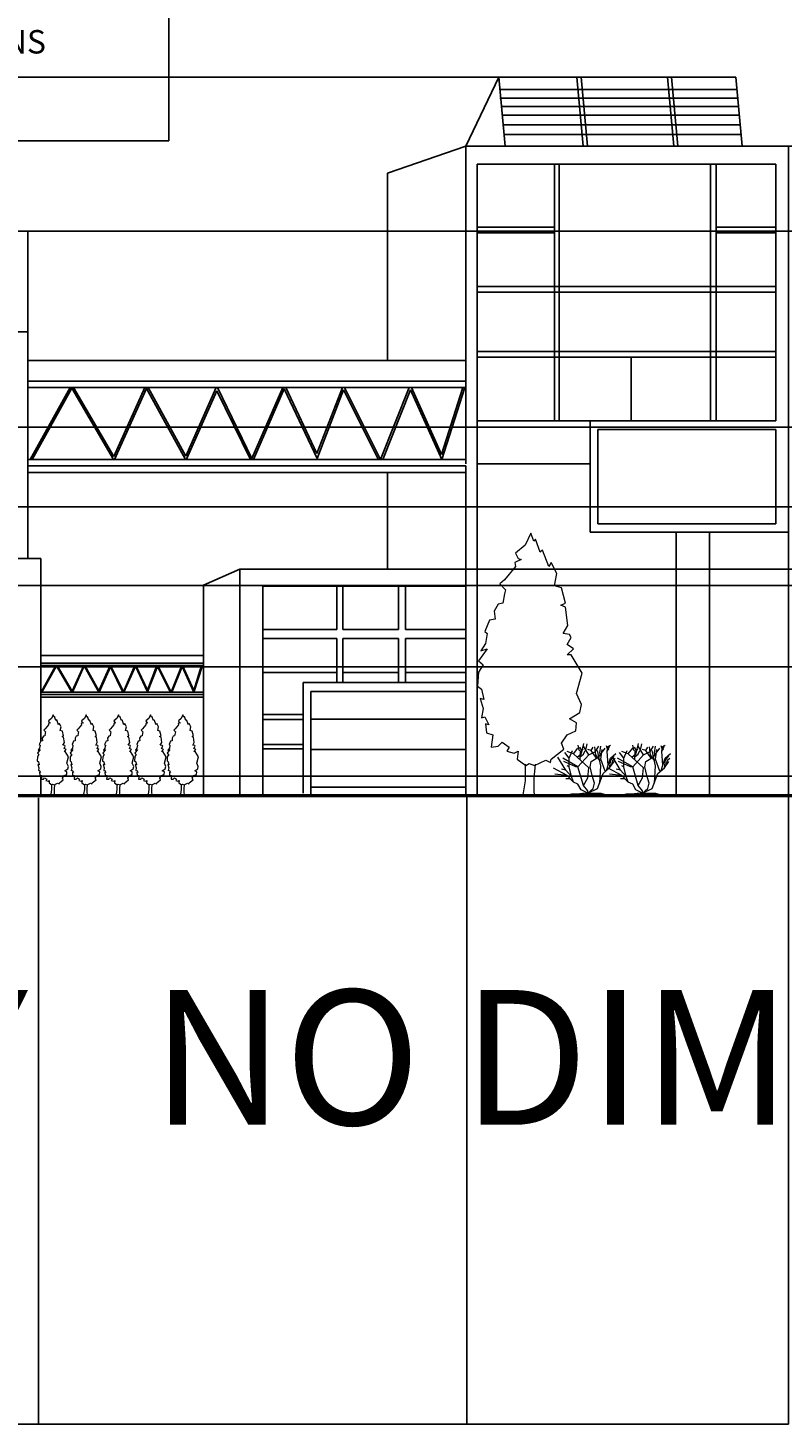
# Model space of a CAD drawing. Units: inches. Extents: x -32109 to 33221, y -19197 to 7608.
# Tile 17 of 25: x 2967 to 6939, y -5430 to 1922. Entities that reach past the tile are written whole.
import ezdxf

# ---------------------------------------------------------------- set-up
doc = ezdxf.new("R2010")
doc.units = ezdxf.units.IN
doc.header["$MEASUREMENT"] = 0
for name, color, linetype, lineweight in [('A-ANNO-DIMS', 2, 'Continuous', 18), ('A-ANNO-TEXT', 7, 'Continuous', 25), ('A-ELEV', 7, 'Continuous', 25), ('L-PLNT', 3, 'Continuous', 13)]:
    doc.layers.add(name, color=color, linetype=linetype, lineweight=lineweight)
doc.styles.get("Standard").update_dxf_attribs({"font": 'arial.ttf'})
doc.dimstyles.get("Standard").update_dxf_attribs({"dimtxt": 0.18, "dimasz": 0.18, "dimexe": 0.18, "dimexo": 0.0625, "dimgap": 0.09, "dimtad": 0, "dimtih": 1, "dimtoh": 1, "dimdec": 4, "dimzin": 0, "dimdsep": 46, "dimtxsty": 'Standard', "dimcen": 0.09, "dimadec": 0, "dimazin": 0, "dimtfac": 1, "dimtdec": 4, "dimtofl": 0, "dimtmove": 0, "dimatfit": 3, "dimfxl": 1, "dimtolj": 1, "dimtzin": 0, "dimarcsym": 0})

# ---------------------------------------------------------------- blocks, each defined once
blk = doc.blocks.new('*U2')
blk.add_lwpolyline([(-2.75400000000036, 191.699), (-6.7800000000002, 182.8509999999996), (-13.68200000000024, 176.9529999999995), (-11.95600000000013, 173.2659999999996), (-9.655999999999949, 172.529), (-14.25700000000006, 170.317), (-13.68200000000024, 167.3679999999999), (-21.73300000000017, 157.7829999999999), (-25.1840000000002, 154.8340000000003), (-21.15800000000036, 150.4099999999998), (-21.73300000000017, 147.4609999999998), (-22.88400000000001, 140.8249999999998), (-26.33400000000029, 140.087), (-29.21000000000004, 134.9259999999995), (-28.63499999999977, 129.0279999999998), (-32.66100000000006, 128.2909999999997), (-36.11099999999988, 120.1799999999998), (-34.38599999999997, 118.7059999999997), (-35.53600000000006, 111.3329999999996), (-38.98700000000008, 106.1709999999998), (-34.38599999999997, 107.6459999999997), (-40.71199999999999, 98.79799999999977), (-37.26099999999997, 95.8489999999997), (-40.71199999999999, 90.68799999999965), (-41.28700000000026, 80.36599999999999), (-38.41200000000026, 78.154), (-36.68600000000015, 70.78099999999995), (-39.5619999999999, 71.51799999999957), (-37.26099999999997, 64.14499999999998), (-38.41200000000026, 57.50899999999956), (-36.11099999999988, 58.24699999999984), (-33.23599999999988, 52.3479999999995), (-35.53600000000006, 53.08599999999978), (-34.96100000000024, 46.44999999999981), (-30.36000000000013, 44.9749999999999), (-31.50999999999977, 36.1279999999997), (-26.33400000000029, 36.86499999999978), (-23.45900000000029, 39.81399999999985), (-18.28300000000036, 36.1279999999997), (-20.00800000000027, 33.17799999999988), (-14.83199999999988, 31.70399999999972), (-11.95600000000013, 33.17799999999988), (-12.53099999999995, 27.27999999999975), (-6.204999999999927, 22.85599999999977), (-3.9050000000002, 24.33099999999968), (0.1209999999996398, 22.85599999999977), (8.172999999999774, 26.54299999999967), (11.62399999999979, 25.06799999999976), (12.19900000000007, 27.27999999999975), (21.40000000000009, 34.6529999999998), (19.67500000000018, 39.07699999999977), (23.70099999999957, 44.9749999999999), (30.02700000000004, 47.92399999999997), (30.60199999999986, 53.82299999999986), (25.42599999999993, 56.77199999999993), (32.90299999999979, 61.19599999999991), (34.05299999999988, 67.0939999999996), (30.60199999999986, 75.20499999999993), (34.6279999999997, 89.95100000000002), (26.57599999999957, 103.2219999999997), (23.70099999999957, 103.2219999999997), (28.30199999999968, 107.6459999999997), (23.70099999999957, 110.5949999999998), (26.57599999999957, 115.7559999999994), (25.42599999999993, 117.9679999999998), (20.82499999999982, 118.7059999999997), (24.27599999999984, 124.6040000000002), (22.55099999999993, 137.8759999999997), (19.09999999999991, 139.3499999999999), (22.55099999999993, 140.8249999999998), (19.67500000000018, 151.884), (14.49899999999979, 153.3589999999999), (16.22400000000016, 162.2069999999999), (12.19900000000007, 170.317), (10.47299999999995, 167.3679999999999), (5.871999999999843, 179.1649999999999), (4.146999999999934, 177.69), (0.6959999999999127, 187.2749999999996), (-0.4540000000001783, 185.7999999999997)], close=True)
for points in [[(-6.813000000000101, 23.66899999999987), (-6.813000000000101, 11.66899999999987), (-8.626999999999953, 0)], [(0.3869999999997162, 23.66899999999987), (-0.5760000000000219, 13.27099999999973), (-0.5760000000000219, 3.685999999999694), (0, 0)]]:
    blk.add_lwpolyline(points)
blk = doc.blocks.new('*U3')
for p, q in [((-16.79999999999995, 16.31999999999993), (-18.7199999999998, 18.7199999999998)), ((-14.87999999999988, 18.24000000000001), (-17.75999999999999, 19.19999999999982)), ((-16.79999999999995, 16.31999999999993), (-15.3599999999999, 19.67999999999983)), ((-14.87999999999988, 18.24000000000001), (-12.95999999999981, 20.63999999999987)), ((-12.47099999999977, 19.77499999999986), (-12.89799999999991, 22.04399999999987)), ((-11.67699999999991, 19.07099999999991), (-12.47099999999977, 19.77499999999986)), ((-11.27999999999997, 19.61899999999991), (-12.10400000000004, 21.18399999999974)), ((-12.04299999999989, 15.6279999999997), (-11.92099999999982, 18.83600000000001)), ((-11.92099999999982, 18.83600000000001), (-10.6400000000001, 20.40100000000007)), ((-11.43299999999999, 18.28899999999976), (-10.45699999999988, 22.7489999999998)), ((-10.57899999999995, 18.05399999999986), (-9.845999999999776, 19.69699999999966)), ((-8.160000000000082, 17.75999999999999), (-10.55999999999994, 21.59999999999991)), ((-9.480000000000018, 19.77499999999986), (-8.991999999999962, 22.59199999999964)), ((-7.200000000000045, 19.67999999999983), (-8.6400000000001, 20.15999999999985)), ((-8.160000000000082, 17.75999999999999), (-5.279999999999972, 19.19999999999982)), ((-7.200000000000045, 19.67999999999983), (-6.240000000000009, 21.11999999999989)), ((-4.799999999999954, 16.31999999999993), (-7.200000000000045, 19.67999999999983)), ((-5.085999999999785, 17.74099999999998), (-5.512999999999919, 21.33999999999992)), ((-5.279999999999972, 19.19999999999982), (-3.840000000000145, 21.59999999999991)), ((-2.880000000000109, 12.95999999999981), (-4.319999999999936, 19.67999999999983)), ((-3.840000000000145, 16.79999999999995), (-0.9600000000000363, 20.63999999999987)), ((-3.376999999999952, 18.60199999999963), (-2.887999999999919, 21.57499999999982)), ((-2.765999999999849, 16.80199999999968), (-3.376999999999952, 18.60199999999963)), ((-2.880000000000109, 15.83999999999992), (-2.40000000000009, 20.15999999999985)), ((-0.5079999999998109, 21.88799999999969), (-0.0809999999999036, 20.55799999999976)), ((-0.2029999999999745, 19.14899999999988), (0.1020000000000891, 21.33999999999992)), ((0.3460000000000036, 13.20299999999974), (-0.2029999999999745, 19.14899999999988)), ((-0.1419999999998254, 19.38399999999979), (0.5899999999999181, 20.40100000000007)), ((-0.0199999999999818, 20.00999999999999), (0.895999999999958, 21.10499999999979)), ((0.04099999999994, 20.71399999999994), (1.384000000000241, 22.04399999999987)), ((0.1020000000000891, 21.33999999999992), (0.8350000000000363, 21.88799999999969)), ((-18.23999999999978, 11.03999999999996), (-21.75499999999988, 16.65499999999997)), ((-12.95999999999981, 12.47999999999979), (-19.67999999999983, 16.31999999999993)), ((-13.91999999999984, 12.47999999999979), (-19.19999999999982, 14.87999999999988)), ((-16.79999999999995, 12.47999999999979), (-17.75999999999999, 12.95999999999981)), ((-16.79999999999995, 12.47999999999979), (-16.79999999999995, 16.31999999999993)), ((-15.83999999999992, 8.159999999999854), (-16.79999999999995, 12.47999999999979)), ((-8.160000000000082, 12), (-14.87999999999988, 18.24000000000001)), ((-12.95999999999981, 12.47999999999979), (-13.91999999999984, 12.47999999999979)), ((-13.32499999999982, 16.72399999999993), (-11.43299999999999, 18.28899999999976)), ((-12.95999999999981, 12.47999999999979), (-8.160000000000082, 17.75999999999999)), ((-10.55999999999994, 4.319999999999936), (-12.95999999999981, 12.47999999999979)), ((-11.98199999999997, 16.80199999999968), (-10.57899999999995, 18.05399999999986)), ((-7.680000000000063, 12.47999999999979), (-7.200000000000045, 14.87999999999988)), ((-6.720000000000027, 8.639999999999873), (-7.680000000000063, 12.47999999999979)), ((-7.200000000000045, 14.87999999999988), (-3.840000000000145, 16.79999999999995)), ((-3.376999999999952, 15.31499999999982), (-5.085999999999785, 17.81899999999973)), ((-3.360000000000127, 5.279999999999972), (-2.880000000000109, 12.95999999999981)), ((-0.9600000000000363, 10.55999999999994), (-2.880000000000109, 15.83999999999992)), ((-0.4800000000000182, 10.79999999999995), (0.3460000000000036, 13.20299999999974)), ((0.3460000000000036, 13.20299999999974), (1.323000000000092, 16.2539999999999)), ((0.9600000000000363, 12), (1.440000000000054, 15.3599999999999)), ((0.9600000000000363, 12), (2.879999999999881, 14.87999999999988)), ((1.323000000000092, 16.2539999999999), (3.642000000000052, 18.28899999999976)), ((1.440000000000054, 15.3599999999999), (2.879999999999881, 17.27999999999997)), ((1.920000000000072, 13.43999999999982), (2.399999999999863, 15.3599999999999)), ((2.399999999999863, 15.3599999999999), (3.359999999999899, 16.31999999999993)), ((-17.75999999999999, 8.639999999999873), (-23.66300000000001, 11.96100000000001)), ((-17.75999999999999, 8.639999999999873), (-23.12799999999993, 9.221999999999753)), ((-18.23999999999978, 11.03999999999996), (-20.15999999999985, 11.51999999999998)), ((-15.83999999999992, 8.159999999999854), (-18.23999999999978, 11.03999999999996)), ((-16.31999999999993, 7.199999999999818), (-18.23999999999978, 7.199999999999818)), ((-14.87999999999988, 5.75999999999999), (-17.75999999999999, 8.639999999999873)), ((-14.87999999999988, 5.75999999999999), (-15.83999999999992, 8.159999999999854)), ((-10.55999999999994, 4.319999999999936), (-8.6400000000001, 7.679999999999836)), ((-8.6400000000001, 7.679999999999836), (-8.160000000000082, 12)), ((-5.75999999999999, 5.279999999999972), (-6.720000000000027, 8.639999999999873)), ((-4.319999999999936, 2.879999999999881), (-1.920000000000072, 9.599999999999909)), ((-1.920000000000072, 9.599999999999909), (0.9600000000000363, 12)), ((-15.83999999999992, 0.4799999999997909), (-17.75999999999999, 0)), ((-13.43999999999982, 0.4799999999997909), (-15.83999999999992, 0.4799999999997909)), ((-12.95999999999981, 4.799999999999954), (-14.87999999999988, 5.75999999999999)), ((-9.600000000000136, 0.959999999999809), (-13.43999999999982, 0.4799999999997909)), ((-11.51999999999998, 2.399999999999863), (-12.95999999999981, 4.799999999999954)), ((-9.600000000000136, 0.959999999999809), (-12.95999999999981, 0)), ((-8.6400000000001, 0.959999999999809), (-11.51999999999998, 2.399999999999863)), ((-8.6400000000001, 1.919999999999845), (-10.55999999999994, 4.319999999999936)), ((-9.600000000000136, 0.959999999999809), (-7.680000000000063, 0.959999999999809)), ((-8.6400000000001, 0.959999999999809), (-4.319999999999936, 2.879999999999881)), ((-8.6400000000001, 0.959999999999809), (-6.240000000000009, 2.879999999999881)), ((-8.6400000000001, 0.959999999999809), (-8.6400000000001, 1.919999999999845)), ((-8.6400000000001, 0.959999999999809), (-2.880000000000109, 0.959999999999809)), ((-7.680000000000063, 0.959999999999809), (-6.240000000000009, 0.4799999999997909)), ((-6.240000000000009, 2.879999999999881), (-5.75999999999999, 5.279999999999972)), ((-6.240000000000009, 0.4799999999997909), (-3.360000000000127, 0)), ((-2.880000000000109, 0.959999999999809), (0, 0))]:
    blk.add_line(p, q)
blk = doc.blocks.new('*D10')
at = {"layer": 'A-ANNO-DIMS', "color": 0, "lineweight": -2, "transparency": 16777216}
for p, q in [((-18512.646816, -110.179138), (-18512.646816, 5772.015489000001)), ((-18512.466816, 5771.835489), (-202.0927503703958, 5771.835489)), ((18109.136745, 5771.835489), (-201.2373206296045, 5771.835489)), ((18109.316745, -101.537382), (18109.316745, 5772.015489000001))]:
    blk.add_line(p, q, dxfattribs=at)
at = {"layer": 'A-ANNO-DIMS', "color": 0, "transparency": 16777216}
for points in [[(-18512.466816, 5771.865488999999), (-18512.466816, 5771.805489000001), (-18512.646816, 5771.835489)], [(18109.136745, 5771.865488999999), (18109.136745, 5771.805489000001), (18109.316745, 5771.835489)]]:
    blk.add_solid(points, dxfattribs=at)
at = {"layer": 'Defpoints', "color": 0, "transparency": 16777216}
for p in [(18109.316745, 5771.835489), (-18512.646816, -110.241638), (18109.316745, -101.599882)]:
    blk.add_point(p, dxfattribs=at)
at = {"layer": 'A-ANNO-DIMS', "color": 0, "transparency": 16777216, "insert": (-201.6650355000002, 5771.835489), "char_height": 0.18, "attachment_point": 5}
blk.add_mtext('\\A1;36622', dxfattribs=at)
blk = doc.blocks.new('*D11')
at = {"layer": 'A-ANNO-DIMS', "color": 0, "lineweight": -2, "transparency": 16777216}
for p, q in [((14509.612941, 1705.161904000001), (25710.64858400003, 1705.161904000003)), ((25710.46858400003, 1704.981904000003), (25710.46858400003, -209.6323674706641)), ((25710.46858400003, -2124.610567999994), (25710.46858400003, -209.9962965293272)), ((-18512.58431600001, -2124.790568000001), (25710.64858400003, -2124.790567999994))]:
    blk.add_line(p, q, dxfattribs=at)
at = {"layer": 'A-ANNO-DIMS', "color": 0, "transparency": 16777216}
for points in [[(25710.43858400003, 1704.981904000003), (25710.49858400002, 1704.981904000003), (25710.46858400003, 1705.161904000003)], [(25710.43858400003, -2124.610567999994), (25710.49858400002, -2124.610567999994), (25710.46858400003, -2124.790567999994)]]:
    blk.add_solid(points, dxfattribs=at)
at = {"layer": 'Defpoints', "color": 0, "transparency": 16777216}
for p in [(14509.550441, 1705.161904000001), (-18512.64681600001, -2124.790568000001), (25710.46858400003, -2124.790567999994)]:
    blk.add_point(p, dxfattribs=at)
at = {"layer": 'A-ANNO-DIMS', "color": 0, "transparency": 16777216, "insert": (25710.46858400002, -209.8143320000029), "char_height": 0.18, "attachment_point": 5}
blk.add_mtext('\\A1;3830', dxfattribs=at)
blk = doc.blocks.new('*D53')
at = {"layer": 'A-ANNO-DIMS', "color": 0, "lineweight": -2, "transparency": 16777216}
for p, q in [((-9508.270603000004, -179.678781), (25710.64858400002, -179.6787809999944)), ((25710.46858400003, -179.8587809999944), (25710.46858400003, -389.7342653622047)), ((25710.46858400003, -599.9735559999946), (25710.46858400003, -390.0980716377845)), ((-9508.270603000004, -600.1535560000002), (25710.64858400002, -600.1535559999945))]:
    blk.add_line(p, q, dxfattribs=at)
at = {"layer": 'A-ANNO-DIMS', "color": 0, "transparency": 16777216}
for points in [[(25710.43858400003, -179.8587809999944), (25710.49858400002, -179.8587809999944), (25710.46858400003, -179.6787809999944)], [(25710.43858400003, -599.9735559999946), (25710.49858400002, -599.9735559999946), (25710.46858400003, -600.1535559999945)]]:
    blk.add_solid(points, dxfattribs=at)
at = {"layer": 'Defpoints', "color": 0, "transparency": 16777216}
for p in [(-9508.333103000004, -179.678781), (-9508.333103000004, -600.1535560000002), (25710.46858400003, -600.1535559999945)]:
    blk.add_point(p, dxfattribs=at)
at = {"layer": 'A-ANNO-DIMS', "color": 0, "transparency": 16777216, "insert": (25710.46858400002, -389.9161685000017), "char_height": 0.18, "attachment_point": 5}
blk.add_mtext('\\A1;420.5', dxfattribs=at)
blk = doc.blocks.new('*D54')
at = {"layer": 'A-ANNO-DIMS', "color": 0, "lineweight": -2, "transparency": 16777216}
for p, q in [((-9508.270603000004, -600.1535560000002), (25710.64858400002, -600.1535559999945)), ((25710.46858400003, -600.3335559999944), (25710.46858400003, -806.8386914706632)), ((25710.46858400003, -1013.707755999995), (25710.46858400003, -807.2026205293262)), ((-9508.270603000004, -1013.887756), (25710.64858400002, -1013.887755999995))]:
    blk.add_line(p, q, dxfattribs=at)
at = {"layer": 'A-ANNO-DIMS', "color": 0, "transparency": 16777216}
for points in [[(25710.43858400003, -600.3335559999944), (25710.49858400002, -600.3335559999944), (25710.46858400003, -600.1535559999945)], [(25710.43858400003, -1013.707755999995), (25710.49858400002, -1013.707755999995), (25710.46858400003, -1013.887755999995)]]:
    blk.add_solid(points, dxfattribs=at)
at = {"layer": 'Defpoints', "color": 0, "transparency": 16777216}
for p in [(-9508.333103000004, -600.1535560000002), (-9508.333103000004, -1013.887756), (25710.46858400003, -1013.887755999995)]:
    blk.add_point(p, dxfattribs=at)
at = {"layer": 'A-ANNO-DIMS', "color": 0, "transparency": 16777216, "insert": (25710.46858400002, -807.0206560000016), "char_height": 0.18, "attachment_point": 5}
blk.add_mtext('\\A1;413.7', dxfattribs=at)
blk = doc.blocks.new('*D55')
at = {"layer": 'A-ANNO-DIMS', "color": 0, "lineweight": -2, "transparency": 16777216}
for p, q in [((-9508.270603000004, -1013.887756), (25710.64858400002, -1013.887755999995)), ((25710.46858400003, -1014.067755999994), (25710.46858400003, -1227.669337362204)), ((25710.46858400003, -1441.634724999994), (25710.46858400003, -1228.033143637784)), ((-9508.270603000004, -1441.814725), (25710.64858400002, -1441.814724999995))]:
    blk.add_line(p, q, dxfattribs=at)
at = {"layer": 'A-ANNO-DIMS', "color": 0, "transparency": 16777216}
for points in [[(25710.43858400003, -1014.067755999994), (25710.49858400002, -1014.067755999994), (25710.46858400003, -1013.887755999995)], [(25710.43858400003, -1441.634724999994), (25710.49858400002, -1441.634724999994), (25710.46858400003, -1441.814724999995)]]:
    blk.add_solid(points, dxfattribs=at)
at = {"layer": 'Defpoints', "color": 0, "transparency": 16777216}
for p in [(-9508.333103000004, -1013.887756), (-9508.333103000004, -1441.814725), (25710.46858400003, -1441.814724999995)]:
    blk.add_point(p, dxfattribs=at)
at = {"layer": 'A-ANNO-DIMS', "color": 0, "transparency": 16777216, "insert": (25710.46858400002, -1227.851240500001), "char_height": 0.18, "attachment_point": 5}
blk.add_mtext('\\A1;427.9', dxfattribs=at)
blk = doc.blocks.new('*D56')
at = {"layer": 'A-ANNO-DIMS', "color": 0, "lineweight": -2, "transparency": 16777216}
for p, q in [((-9508.270603000004, -1441.814725), (25710.64858400002, -1441.814724999995)), ((25710.46858400003, -1441.994724999995), (25710.46858400003, -1730.102620862205)), ((25710.46858400003, -2018.574322999995), (25710.46858400003, -1730.466427137785)), ((-9508.270603000004, -2018.754323000001), (25710.64858400002, -2018.754322999996))]:
    blk.add_line(p, q, dxfattribs=at)
at = {"layer": 'A-ANNO-DIMS', "color": 0, "transparency": 16777216}
for points in [[(25710.43858400003, -1441.994724999995), (25710.49858400002, -1441.994724999995), (25710.46858400003, -1441.814724999995)], [(25710.43858400003, -2018.574322999995), (25710.49858400002, -2018.574322999995), (25710.46858400003, -2018.754322999996)]]:
    blk.add_solid(points, dxfattribs=at)
at = {"layer": 'Defpoints', "color": 0, "transparency": 16777216}
for p in [(-9508.333103000004, -1441.814725), (-9508.333103000004, -2018.754323000001), (25710.46858400003, -2018.754322999996)]:
    blk.add_point(p, dxfattribs=at)
at = {"layer": 'A-ANNO-DIMS', "color": 0, "transparency": 16777216, "insert": (25710.46858400002, -1730.284524000002), "char_height": 0.18, "attachment_point": 5}
blk.add_mtext('\\A1;576.9', dxfattribs=at)
blk = doc.blocks.new('*D57')
at = {"layer": 'A-ANNO-DIMS', "color": 0, "lineweight": -2, "transparency": 16777216}
for p, q in [((1588.180692, -2116.211312), (1588.180692, -5429.734913)), ((3022.7376, -2131.466103000001), (3022.7376, -5429.734913)), ((1588.360692, -5429.554913), (2305.004050502047, -5429.554913)), ((3022.5576, -5429.554913), (2305.914241497954, -5429.554913))]:
    blk.add_line(p, q, dxfattribs=at)
at = {"layer": 'A-ANNO-DIMS', "color": 0, "transparency": 16777216}
for points in [[(1588.360692, -5429.524913), (1588.360692, -5429.584913), (1588.180692, -5429.554913)], [(3022.5576, -5429.524913), (3022.5576, -5429.584913), (3022.7376, -5429.554913)]]:
    blk.add_solid(points, dxfattribs=at)
at = {"layer": 'Defpoints', "color": 0, "transparency": 16777216}
for p in [(1588.180692, -2116.148812), (3022.7376, -2131.403603), (3022.7376, -5429.554913)]:
    blk.add_point(p, dxfattribs=at)
at = {"layer": 'A-ANNO-DIMS', "color": 0, "transparency": 16777216, "insert": (2305.459146, -5429.554913), "char_height": 0.18, "attachment_point": 5}
blk.add_mtext('\\A1;1434.6', dxfattribs=at)
blk = doc.blocks.new('*D58')
at = {"layer": 'A-ANNO-DIMS', "color": 0, "lineweight": -2, "transparency": 16777216}
for p, q in [((3022.7376, -2131.466103000001), (3022.7376, -5429.734913)), ((5279.264054, -2122.811479), (5279.264054, -5429.734913)), ((3022.9176, -5429.554913), (4150.534987982264, -5429.554913)), ((5279.084054, -5429.554913), (4151.466666017735, -5429.554913))]:
    blk.add_line(p, q, dxfattribs=at)
at = {"layer": 'A-ANNO-DIMS', "color": 0, "transparency": 16777216}
for points in [[(3022.9176, -5429.524913), (3022.9176, -5429.584913), (3022.7376, -5429.554913)], [(5279.084054, -5429.524913), (5279.084054, -5429.584913), (5279.264054, -5429.554913)]]:
    blk.add_solid(points, dxfattribs=at)
at = {"layer": 'Defpoints', "color": 0, "transparency": 16777216}
for p in [(3022.7376, -2131.403603), (5279.264054, -2122.748979), (5279.264054, -5429.554913)]:
    blk.add_point(p, dxfattribs=at)
at = {"layer": 'A-ANNO-DIMS', "color": 0, "transparency": 16777216, "insert": (4151.000826999999, -5429.554913), "char_height": 0.18, "attachment_point": 5}
blk.add_mtext('\\A1;2256.5', dxfattribs=at)
blk = doc.blocks.new('*D59')
at = {"layer": 'A-ANNO-DIMS', "color": 0, "lineweight": -2, "transparency": 16777216}
for p, q in [((6972.547547000001, 1298.608475), (6972.547547000001, -5429.734913)), ((5279.264054, -2122.811479), (5279.264054, -5429.734913)), ((5279.444054, -5429.554913), (6125.450643610506, -5429.554913)), ((6972.367547000001, -5429.554913), (6126.360957389495, -5429.554913))]:
    blk.add_line(p, q, dxfattribs=at)
at = {"layer": 'A-ANNO-DIMS', "color": 0, "transparency": 16777216}
for points in [[(5279.444054, -5429.524913), (5279.444054, -5429.584913), (5279.264054, -5429.554913)], [(6972.367547000001, -5429.524913), (6972.367547000001, -5429.584913), (6972.547547000001, -5429.554913)]]:
    blk.add_solid(points, dxfattribs=at)
at = {"layer": 'Defpoints', "color": 0, "transparency": 16777216}
for p in [(6972.547547000001, 1298.670975), (5279.264054, -2122.748979), (6972.547547000001, -5429.554913)]:
    blk.add_point(p, dxfattribs=at)
at = {"layer": 'A-ANNO-DIMS', "color": 0, "transparency": 16777216, "insert": (6125.9058005, -5429.554913), "char_height": 0.18, "attachment_point": 5}
blk.add_mtext('\\A1;1693.3', dxfattribs=at)
blk = doc.blocks.new('*D67')
at = {"layer": 'A-ANNO-DIMS', "color": 0, "lineweight": -2, "transparency": 16777216}
for p, q in [((1645.907271000001, 851.2050040000005), (25710.64858400003, 851.2050040000044)), ((25710.46858400003, 851.0250040000043), (25710.46858400003, -632.2900008622063)), ((25710.46858400003, -2115.968811999997), (25710.46858400003, -632.6538071377862)), ((1588.243192000001, -2116.148812000001), (25710.64858400003, -2116.148811999997))]:
    blk.add_line(p, q, dxfattribs=at)
at = {"layer": 'A-ANNO-DIMS', "color": 0, "transparency": 16777216}
for points in [[(25710.43858400003, 851.0250040000043), (25710.49858400002, 851.0250040000043), (25710.46858400003, 851.2050040000044)], [(25710.43858400003, -2115.968811999997), (25710.49858400002, -2115.968811999997), (25710.46858400003, -2116.148811999997)]]:
    blk.add_solid(points, dxfattribs=at)
at = {"layer": 'Defpoints', "color": 0, "transparency": 16777216}
for p in [(1645.844771000001, 851.2050040000005), (1588.180692, -2116.148812000001), (25710.46858400003, -2116.148811999997)]:
    blk.add_point(p, dxfattribs=at)
at = {"layer": 'A-ANNO-DIMS', "color": 0, "transparency": 16777216, "insert": (25710.46858400002, -632.4719040000035), "char_height": 0.18, "attachment_point": 5}
blk.add_mtext('\\A1;2967.4', dxfattribs=at)
blk = doc.blocks.new('*D68')
at = {"layer": 'A-ANNO-DIMS', "color": 0, "lineweight": -2, "transparency": 16777216}
for p, q in [((4084.059477000002, -927.4788990000004), (25710.64858400003, -927.478898999997)), ((25710.46858400003, -927.658898999997), (25710.46858400003, -1521.631952362207)), ((25710.46858400003, -2115.968811999997), (25710.46858400003, -1521.995758637787)), ((4084.059477000002, -2116.148812000001), (25710.64858400003, -2116.148811999997))]:
    blk.add_line(p, q, dxfattribs=at)
at = {"layer": 'A-ANNO-DIMS', "color": 0, "transparency": 16777216}
for points in [[(25710.43858400003, -927.658898999997), (25710.49858400002, -927.658898999997), (25710.46858400003, -927.478898999997)], [(25710.43858400003, -2115.968811999997), (25710.49858400002, -2115.968811999997), (25710.46858400003, -2116.148811999997)]]:
    blk.add_solid(points, dxfattribs=at)
at = {"layer": 'Defpoints', "color": 0, "transparency": 16777216}
for p in [(4083.996977000001, -927.4788990000004), (4083.996977000001, -2116.148812000001), (25710.46858400003, -2116.148811999997)]:
    blk.add_point(p, dxfattribs=at)
at = {"layer": 'A-ANNO-DIMS', "color": 0, "transparency": 16777216, "insert": (25710.46858400002, -1521.813855500004), "char_height": 0.18, "attachment_point": 5}
blk.add_mtext('\\A1;1188.7', dxfattribs=at)
blk = doc.blocks.new('*D69')
at = {"layer": 'A-ANNO-DIMS', "color": 0, "lineweight": -2, "transparency": 16777216}
for p, q in [((5273.811589000001, 1298.670975), (25710.64858400003, 1298.670975000004)), ((25710.46858400003, 1298.490975000003), (25710.46858400003, -411.8570374706656)), ((25710.46858400003, -2122.568978999998), (25710.46858400003, -412.2209665293287)), ((5279.326554000002, -2122.748979000001), (25710.64858400003, -2122.748978999998))]:
    blk.add_line(p, q, dxfattribs=at)
at = {"layer": 'A-ANNO-DIMS', "color": 0, "transparency": 16777216}
for points in [[(25710.43858400003, 1298.490975000003), (25710.49858400002, 1298.490975000003), (25710.46858400003, 1298.670975000004)], [(25710.43858400003, -2122.568978999998), (25710.49858400002, -2122.568978999998), (25710.46858400003, -2122.748978999998)]]:
    blk.add_solid(points, dxfattribs=at)
at = {"layer": 'Defpoints', "color": 0, "transparency": 16777216}
for p in [(5273.749089000002, 1298.670975), (5279.264054000002, -2122.748979000001), (25710.46858400003, -2122.748978999998)]:
    blk.add_point(p, dxfattribs=at)
at = {"layer": 'A-ANNO-DIMS', "color": 0, "transparency": 16777216, "insert": (25710.46858400002, -412.0390020000043), "char_height": 0.18, "attachment_point": 5}
blk.add_mtext('\\A1;3421.4', dxfattribs=at)
blk = doc.blocks.new('*D158')
at = {"layer": 'A-ANNO-DIMS', "color": 0, "lineweight": -2, "transparency": 16777216}
for p, q in [((5447.266114000002, 1662.169531000001), (-24361.99565300002, 1662.169530999996)), ((-24361.81565300002, 1661.989530999996), (-24361.81565300002, -230.1077594706735)), ((-24361.81565300002, -2122.568979000006), (-24361.81565300002, -230.4716885293365)), ((5279.201554000002, -2122.748979000001), (-24361.99565300002, -2122.748979000006))]:
    blk.add_line(p, q, dxfattribs=at)
at = {"layer": 'A-ANNO-DIMS', "color": 0, "transparency": 16777216}
for points in [[(-24361.84565300001, 1661.989530999996), (-24361.78565300002, 1661.989530999996), (-24361.81565300002, 1662.169530999996)], [(-24361.84565300001, -2122.568979000006), (-24361.78565300002, -2122.568979000006), (-24361.81565300002, -2122.748979000006)]]:
    blk.add_solid(points, dxfattribs=at)
at = {"layer": 'Defpoints', "color": 0, "transparency": 16777216}
for p in [(5447.328614000002, 1662.169531000001), (-24361.81565300002, -2122.748979000006), (5279.264054000002, -2122.748979000001)]:
    blk.add_point(p, dxfattribs=at)
at = {"layer": 'A-ANNO-DIMS', "color": 0, "transparency": 16777216, "insert": (-24361.81565300001, -230.289723999998), "char_height": 0.18, "attachment_point": 5}
blk.add_mtext('\\A1;3784.9', dxfattribs=at)

msp = doc.modelspace()

# ---------------------------------------------------------------- linework, layer by layer
at = {"layer": 'A-ELEV'}
for p, q in [((3709.007830620743, 2649.474070118566), (3709.007830620743, 1327.301250283199)), ((5447.32861392136, 1662.169530563798), (5273.749089065008, 1298.670974604101)), ((5480.666080008848, 1298.670974604102), (5447.32861392136, 1662.169530563798)), ((5447.32861392136, 1662.169530563798), (6694.540015472156, 1662.169530563798)), ((5890.710555356229, 1298.670974604102), (5857.373089268742, 1662.169530563798)), ((5890.710555356229, 1298.670974604102), (5857.373089268742, 1662.169530563798)), ((5914.211863851466, 1298.670974604102), (5880.874397763978, 1662.169530563798)), ((6368.346267121845, 1298.670974604102), (6335.008801034357, 1662.169530563798)), ((6390.352765497636, 1298.670974604102), (6357.015299410148, 1662.169530563798)), ((6727.877481559644, 1298.670974604102), (6694.540015472156, 1662.169530563798)), ((5453.256710090786, 1597.531912590028), (6700.468111641583, 1597.531912590028)), ((5453.256710090786, 1552.776496671184), (6704.572755624245, 1552.776496671184)), ((5461.466004493717, 1508.021010559198), (6708.677406044514, 1508.021010559198)), ((5465.570654913987, 1463.265524447211), (6712.782056464785, 1463.265524447212)), ((5470.261681206746, 1412.116427544868), (6717.473082757544, 1412.116427544868)), ((3709.007830620743, 1327.301250283199), (2289.325426198426, 1327.301250283199)), ((5474.952707499508, 1360.96733064251), (6722.164109050307, 1360.96733064251)), ((5273.749089065008, 1298.670974604101), (4861.137779108801, 1157.703068119052)), ((5273.749089065008, 714.3486125170785), (5273.749089065008, 1298.670974604101)), ((5273.749089065008, 1298.670974604101), (6972.547546968148, 1298.670974604101)), ((5333.877798294634, -373.7912973593755), (5333.877798294634, 1203.799654430364)), ((5333.877798294634, 1203.799654430364), (6905.253727797994, 1203.799654430364)), ((5333.877798294633, 1203.799654430364), (6905.253727797995, 1203.799654430364)), ((5741.05250553691, 1203.799654430364), (5741.052505536912, -147.8993357819271)), ((5765.775805699439, 1203.799654430364), (5765.77580569944, -147.8993357819271)), ((6562.417986700229, 1203.799654430364), (6562.417986700229, -147.8993357819271)), ((6592.497502408591, 1203.799654430364), (6592.497502408591, -147.8993357819272)), ((6905.253727797994, 1203.799654430364), (6905.25372779799, -147.8993357819271)), ((4861.137779108801, 170.8274683298532), (4861.137779108801, 1157.703068119052)), ((2967.282875926691, 851.2050040502659), (1645.844771085678, 851.2050040502659)), ((2967.282875926691, 322.0173392160969), (2967.282875926691, 851.2050040502659)), ((5333.877798294633, 872.8815565110854), (5741.052505536909, 872.8815565110856)), ((5333.877798294633, 842.3881196846195), (5741.052505536909, 842.3881196846195)), ((6592.497502408591, 872.8815565110854), (6905.253727797995, 872.8815565110854)), ((6592.497502408591, 842.3881196846194), (6905.253727797995, 842.3881196846195)), ((5273.749089065008, 714.3486125170785), (5273.749089065008, 124.3148270016519)), ((5333.877798294633, 560.9596032502596), (6905.253727797995, 560.9596032502596)), ((5333.877798294633, 530.4661664237937), (6905.253727797995, 530.4661664237937)), ((1645.844771085678, 322.0173392160969), (2967.282875926691, 322.0173392160969)), ((2967.282875926691, -871.5754161552333), (2967.282875926691, 322.0173392160969)), ((2967.238219835289, 170.8274683298532), (5273.749089065008, 170.8274683298532)), ((5333.877798294633, 218.2707407562558), (6905.253727797995, 218.2707407562558)), ((5333.877798294633, 187.7773039297899), (6905.253727797995, 187.7773039297899)), ((6143.985851457318, 187.7773039297899), (6143.985851457318, -147.8993357819272)), ((5273.749089065008, 124.3148270016519), (5273.749089065008, -373.7912973593755)), ((2967.238219835289, 61.3590517298162), (5273.749089065008, 61.3590517298162)), ((2967.238219835289, 28.63557572773789), (5273.749089065008, 28.63557572773789)), ((2978.568256870756, -350.9477259432133), (3190.289100876924, 28.63557572773788)), ((2990.018625116755, -350.9477259432133), (3199.180111183677, 24.04703584496621)), ((3199.180111183677, 24.04703584496618), (3417.192100084115, -350.9477259432133)), ((3208.079629672329, 28.63557572773788), (3419.558679207804, -335.1221066076253)), ((3419.558679207805, -335.1221066076247), (3583.416212694968, 28.63557572773787)), ((3423.626547475391, -350.4395587456416), (3592.27986823659, 23.96459450046246)), ((3592.279868236591, 23.96459450046237), (3796.233585120079, -350.9477259432133)), ((3601.122773337108, 28.63557572773788), (3798.029464996312, -333.3227440758293)), ((3798.029464996312, -333.3227440758297), (3959.325369968427, 28.63557572773787)), ((3802.037490575223, -348.8963902013148), (3962.552740071702, 11.31008882021176)), ((3962.552740071703, 11.31008882021189), (4138.657516396396, -350.9477259432133)), ((3965.249290809271, 28.63557572773787), (4146.800582883963, -344.8260401752486)), ((4146.800582883963, -344.8260401752486), (4309.842380304966, 28.63557572773788)), ((4155.039471919471, -350.9477259432133), (4317.325080345038, 20.78177237623948)), ((4317.325080345039, 20.78177237624018), (4489.707210177424, -344.8260401752486)), ((4324.677854371048, 28.63557572773789), (4488.810927035266, -319.4766892875965)), ((4488.810927035266, -319.4766892875963), (4623.790551185827, 28.63557572773789)), ((4489.707210177424, -344.826040175249), (4629.636371915792, 16.05107547077986)), ((4629.636371915792, 16.05107547077858), (4813.519695872872, -350.9477259432133)), ((4634.515979115877, 28.63557572773789), (4824.704718046174, -350.9477259432133)), ((4824.704718046174, -350.9477259432133), (4975.607651142916, 28.901836342553)), ((4835.464939497505, -350.9477259432133), (4981.31891068586, 16.19269986957999)), ((4981.31891068586, 16.19269986957977), (5146.305278169035, -350.9477259432133)), ((4986.690626181292, 28.63557572773789), (5145.541995599523, -324.852777878823)), ((5145.541995599523, -324.8527778788229), (5257.725422702501, 28.63557572773789)), ((5147.751987027495, -350.9477259432133), (5268.185260021895, 28.5357725521717)), ((5273.749089065008, 28.63557572773789), (5273.749089065008, 61.3590517298162)), ((5928.837878805931, -147.8993357819271), (5333.877798294634, -147.899335781927)), ((5928.837878805931, -147.8993357819271), (5928.837878805932, -732.6545007896601)), ((5928.837878805931, -147.8993357819271), (6905.253727797994, -147.8993357819271)), ((6905.311906553343, -191.9713657656083), (5968.678916879948, -191.9713657656083)), ((5968.678916879948, -191.9713657656083), (5968.678916879948, -689.7670309626427)), ((6905.253727797992, -191.9713657656084), (6905.253727797992, -689.7670309626427)), ((2967.238219835289, -350.9477259432133), (5241.172826178186, -350.9477259432133)), ((5241.172826178186, -350.9477259432133), (5273.749089065008, -350.9477259432133)), ((5241.172826178186, -383.1896425231262), (2967.238219835289, -383.1896425231262)), ((2967.238219835289, -420.0202477263083), (5273.749089065008, -420.0202477263083)), ((4861.137779108802, -420.0202477263082), (4861.137779108801, -927.478899009526)), ((5241.172826178186, -383.1896425231262), (5273.749089065008, -383.1896425231262)), ((5273.749089065008, -383.1896425231262), (5273.749089065008, -2116.148811955302)), ((5333.877798294634, -373.7912973593755), (5333.877798294634, -2116.148811955302)), ((5333.877798294634, -373.7912973593755), (5928.837878805932, -373.7912973593756)), ((5928.837878805932, -732.6545007896601), (6972.547546968148, -732.6545007896601)), ((5968.678916879948, -689.7670309626427), (6905.253727797992, -689.7670309626427)), ((6381.013047934917, -732.65450078966), (6381.013047934917, -2116.148811955302)), ((6557.277818646689, -732.65450078966), (6557.277818646689, -2116.148811955302)), ((1588.180691889405, -871.5754161552333), (3034.293504197781, -871.5754161552333)), ((3034.293504197781, -871.5754161552333), (3034.293504197781, -1833.960081423007)), ((4083.996976847411, -927.4788990095258), (3891.022902107157, -1012.922039376535)), ((4083.996976847411, -927.4788990095258), (4083.996976847411, -2116.148811955302)), ((5273.749089065008, -927.4788990095258), (4083.996976847411, -927.4788990095258)), ((3891.022902107157, -1012.922039376535), (3891.022902107157, -1382.605692586803)), ((4204.670489915646, -2116.148811955302), (4204.670489915646, -1018.541911373424)), ((4204.670489915646, -1018.541911373424), (5273.749089065007, -1018.541911373424)), ((4594.619487114483, -1246.617056267715), (4594.619487114483, -1018.541911373424)), ((4625.853160851722, -1246.617056267715), (4625.853160851722, -1018.541911373424)), ((4918.968498044036, -1246.617056267714), (4918.968498044036, -1018.541911373424)), ((4955.007154641208, -1246.617056267714), (4955.007154641208, -1018.541911373424)), ((4204.670489915646, -1246.617056267714), (4594.619487114484, -1246.617056267714)), ((4625.853160851723, -1246.617056267714), (4918.968498044035, -1246.617056267714)), ((4955.007154641208, -1246.617056267714), (5273.749089065008, -1246.617056267714)), ((4204.670489915646, -1292.53100967966), (4594.619487114485, -1292.53100967966)), ((4594.619487114483, -1524.327302597012), (4594.619487114484, -1292.53100967966)), ((4625.853160851722, -1524.327302597012), (4625.853160851723, -1292.53100967966)), ((4625.853160851723, -1292.53100967966), (4918.968498044036, -1292.53100967966)), ((4918.968498044036, -1524.327302597012), (4918.968498044036, -1292.53100967966)), ((4955.007154641208, -1524.327302597012), (4955.007154641208, -1292.53100967966)), ((4955.007154641208, -1292.53100967966), (5273.749089065008, -1292.53100967966)), ((3034.293504197781, -1382.605692586806), (3891.022902107158, -1382.605692586806)), ((3891.022902107157, -1382.605692586806), (3891.022902107157, -2116.148811955302)), ((3034.293504197781, -1423.224334052506), (3891.022902107158, -1423.224334052506)), ((3034.293504197781, -1435.366495056773), (3891.022902107158, -1435.366495056773)), ((3036.403376190263, -1576.212215820891), (3114.963140920605, -1435.366495056773)), ((3040.652075649705, -1576.212215820891), (3118.262181604069, -1437.069088938535)), ((3118.262181604069, -1437.069088938535), (3199.156297801307, -1576.212215820891)), ((3121.564379278386, -1435.366495056773), (3200.034425318913, -1570.340064037482)), ((3200.034425318913, -1570.340064037482), (3260.834340133492, -1435.366495056773)), ((3201.543822164348, -1576.023658592754), (3264.123230735025, -1437.099679089725)), ((3264.123230735025, -1437.099679089726), (3339.800975595038, -1576.212215820891)), ((3267.404421812315, -1435.366495056773), (3340.467343147195, -1569.672404233716)), ((3340.467343147195, -1569.672404233716), (3400.316756680648, -1435.366495056773)), ((3341.954535152264, -1575.451060470208), (3401.514283722452, -1441.795177984441)), ((3401.514283722452, -1441.795177984441), (3466.858581119805, -1576.212215820891)), ((3402.514848369364, -1435.366495056773), (3469.880094615322, -1573.940742759551)), ((3469.880094615322, -1573.940742759551), (3530.377327689985, -1435.366495056773)), ((3472.937163404685, -1576.212215820891), (3533.15380988972, -1438.28067644703)), ((3533.153809889721, -1438.280676447029), (3597.116806197032, -1573.940742759551)), ((3535.88208258441, -1435.366495056773), (3596.784237180929, -1564.534776846517)), ((3596.784237180929, -1564.534776846517), (3646.86890204439, -1435.366495056773)), ((3597.116806197032, -1573.940742759551), (3649.038014411939, -1440.036018192657)), ((3649.038014411939, -1440.036018192657), (3717.268569299962, -1576.212215820891)), ((3650.848609846764, -1435.366495056773), (3721.418811164729, -1576.212215820891)), ((3721.418811164729, -1576.212215820891), (3777.411875885618, -1435.267698118026)), ((3725.4114292257, -1576.212215820891), (3779.531058850874, -1439.983467960761)), ((3779.531058850874, -1439.983467960761), (3840.749831494791, -1576.212215820891)), ((3781.524252801618, -1435.366495056773), (3840.466612809521, -1566.529593449854)), ((3840.466612809521, -1566.529593449854), (3882.09266848308, -1435.366495056773)), ((3841.28663791122, -1576.212215820891), (3885.97382795411, -1435.403527376518)), ((4204.670489915646, -1472.360526006276), (4594.619487114484, -1472.360526006276)), ((4417.518268981424, -2107.830379083767), (4417.518268981424, -1524.327302597012)), ((4417.518268981424, -1524.327302597012), (5273.749089065008, -1524.327302597012)), ((4625.853160851722, -1472.360526006276), (4918.968498044036, -1472.360526006276)), ((4955.007154641208, -1472.360526006276), (5273.749089065008, -1472.360526006275)), ((3034.293504197781, -1576.212215820891), (3875.950769253788, -1576.212215820891)), ((3875.950769253788, -1588.175692505783), (3034.293504197781, -1588.175692505783)), ((3034.293504197781, -1601.841818263121), (3891.022902107158, -1601.841818263121)), ((3841.286637911219, -1576.212215820891), (3888.038306313237, -1576.212215820891)), ((3875.950769253788, -1588.175692505783), (3891.022902107157, -1588.175692505783)), ((4457.980219635035, -2116.148811955302), (4457.980219635035, -1572.064031023823)), ((4457.980219635035, -1572.064031023823), (5273.749089065008, -1572.064031023823)), ((4417.518268981424, -1694.277768616797), (4204.670489915646, -1694.277768616797)), ((4417.518268981424, -1720.09894060521), (4204.670489915646, -1720.09894060521)), ((4457.980219635035, -1717.234710226214), (5273.749089065008, -1717.234710226214)), ((4417.518268981424, -1850.859603419056), (4204.670489915646, -1850.859603419056)), ((4417.518268981424, -1873.666682711133), (4204.670489915646, -1873.666682711133)), ((4457.980219635035, -1877.933441878326), (5273.749089065008, -1877.933441878326)), ((3034.293504197781, -2013.656842478098), (3034.293504197781, -2116.148811955302)), ((3034.293504197781, -2116.148811955302), (1588.180691889405, -2116.148811955302)), ((3034.29350419778, -2116.148811955302), (9873.79349638903, -2116.148811955302)), ((4083.996976847411, -2116.148811955302), (4204.670489915646, -2116.148811955302)), ((4457.980219635035, -2076.89374287946), (5273.749089065008, -2076.89374287946)), ((5273.749089065008, -2116.148811955302), (5333.877798294634, -2116.148811955302))]:
    msp.add_line(p, q, dxfattribs=at)

# ---------------------------------------------------------------- block references
at = {"layer": 'L-PLNT'}
for name, p, xscale, yscale, zscale in [('*U2', (5634.928582253087, -2127.10446931088), 7.247071498988421, 7.247071498988421, 7.247071498988421), ('*U2', (3105.950065459345, -2113.641820326435), 2.18525868090991, 2.18525868090991, 2.18525868090991), ('*U2', (3279.178399845247, -2113.641820326435), 2.18525868090991, 2.18525868090991, 2.18525868090991), ('*U2', (3450.156991759565, -2113.641820326435), 2.18525868090991, 2.18525868090991, 2.18525868090991), ('*U2', (3618.885841202328, -2113.641820326435), 2.18525868090991, 2.18525868090991, 2.18525868090991), ('*U2', (3789.864433116646, -2113.641820326435), 2.18525868090991, 2.18525868090991, 2.18525868090991), ('*U3', (6019.338550198607, -2118.430999141933), 11.97885450539613, 11.97885450539613, 11.97885450539613), ('*U3', (6307.329269991825, -2118.430999141933), 11.97885450539613, 11.97885450539613, 11.97885450539613)]:
    msp.add_blockref(name, p, dxfattribs=dict(at, xscale=xscale, yscale=yscale, zscale=zscale))

# ---------------------------------------------------------------- texts
at = {"layer": 'A-ANNO-TEXT'}
for s, height, p in [('SKYBRIE   CONNECTIONS', 123.5547426012344, (1102.672851028386, 1787.079753092934)), ('MONUMENTAL    FRONT   FACADE    ( CONCEPTUAL ONLY   NO DIMENSIONS )', 709.7949465747753, (-22238.10681632875, -3853.851877923695))]:
    msp.add_text(s, height=height, dxfattribs=at).set_placement(p)

# ---------------------------------------------------------------- dimensions: what is measured, and where the dimension line sits
at = {"layer": 'A-ANNO-DIMS'}
for base, p1, p2, override, picture, middle in [((18109.316745, 5771.835489), (-18512.646816, -110.241638), (18109.316745, -101.599882), {"dimdec": 0, "dimlfac": 1, "dimrnd": 0, "dimzin": 0, "dimdsep": 46, "dimlunit": 2}, '*D10', (-201.6650355000002, 5771.835489)), ((6972.547547000001, -5429.554913), (5279.264054, -2122.748979), (6972.547547000001, 1298.670975), {"dimdec": 1, "dimlfac": 1, "dimrnd": 0, "dimzin": 0, "dimdsep": 46, "dimlunit": 2}, '*D59', (6125.9058005, -5429.554913)), ((3022.7376, -5429.554913), (1588.180692, -2116.148812), (3022.7376, -2131.403603), {"dimdec": 1, "dimlfac": 1, "dimrnd": 0, "dimzin": 0, "dimdsep": 46, "dimlunit": 2}, '*D57', (2305.459146, -5429.554913)), ((5279.264054, -5429.554913), (3022.7376, -2131.403603), (5279.264054, -2122.748979), {"dimdec": 1, "dimlfac": 1, "dimrnd": 0, "dimzin": 0, "dimdsep": 46, "dimlunit": 2}, '*D58', (4151.000826999999, -5429.554913))]:
    dim = msp.add_linear_dim(base=base, p1=p1, p2=p2, dimstyle='Standard', override=override, dxfattribs=at)
    dim.commit()
    dim.dimension.update_dxf_attribs({"geometry": picture, "text_midpoint": middle})
for base, p1, p2, override, picture, middle in [((25710.46858400003, -2124.790567999994), (14509.550441, 1705.161904), (-18512.646816, -2124.790568), {"dimdec": 0, "dimlfac": 1, "dimrnd": 0, "dimzin": 0, "dimdsep": 46, "dimlunit": 2}, '*D11', (25710.46858400002, -209.8143320000029)), ((-24361.81565300002, -2122.748979000006), (5447.328613999999, 1662.169531), (5279.264054, -2122.748979), {"dimdec": 1, "dimlfac": 1, "dimrnd": 0, "dimzin": 0, "dimdsep": 46, "dimlunit": 2}, '*D158', (-24361.81565300001, -230.289723999998)), ((25710.46858400003, -2122.748978999998), (5273.749089, 1298.670975), (5279.264054, -2122.748979), {"dimdec": 1, "dimlfac": 1, "dimrnd": 0, "dimzin": 0, "dimdsep": 46, "dimlunit": 2}, '*D69', (25710.46858400002, -412.0390020000043)), ((25710.46858400003, -2116.148811999997), (1645.844771, 851.205004), (1588.180692, -2116.148812), {"dimdec": 1, "dimlfac": 1, "dimrnd": 0, "dimzin": 0, "dimdsep": 46, "dimlunit": 2}, '*D67', (25710.46858400002, -632.4719040000035)), ((25710.46858400003, -600.1535559999945), (-9508.333103, -179.678781), (-9508.333103, -600.1535559999999), {"dimdec": 1, "dimlfac": 1, "dimrnd": 0, "dimzin": 0, "dimdsep": 46, "dimlunit": 2}, '*D53', (25710.46858400002, -389.9161685000017)), ((25710.46858400003, -1013.887755999995), (-9508.333103, -600.1535559999999), (-9508.333103, -1013.887756), {"dimdec": 1, "dimlfac": 1, "dimrnd": 0, "dimzin": 0, "dimdsep": 46, "dimlunit": 2}, '*D54', (25710.46858400002, -807.0206560000016)), ((25710.46858400003, -2116.148811999997), (4083.996976999999, -927.478899), (4083.996976999999, -2116.148812), {"dimdec": 1, "dimlfac": 1, "dimrnd": 0, "dimzin": 0, "dimdsep": 46, "dimlunit": 2}, '*D68', (25710.46858400002, -1521.813855500004)), ((25710.46858400003, -1441.814724999995), (-9508.333103, -1013.887756), (-9508.333103, -1441.814725), {"dimdec": 1, "dimlfac": 1, "dimrnd": 0, "dimzin": 0, "dimdsep": 46, "dimlunit": 2}, '*D55', (25710.46858400002, -1227.851240500001)), ((25710.46858400003, -2018.754322999996), (-9508.333103, -1441.814725), (-9508.333103, -2018.754323), {"dimdec": 1, "dimlfac": 1, "dimrnd": 0, "dimzin": 0, "dimdsep": 46, "dimlunit": 2}, '*D56', (25710.46858400002, -1730.284524000002))]:
    dim = msp.add_linear_dim(base=base, p1=p1, p2=p2, angle=90, dimstyle='Standard', override=override, dxfattribs=at)
    dim.commit()
    dim.dimension.update_dxf_attribs({"geometry": picture, "text_midpoint": middle})

doc.saveas('drawing.dxf')
